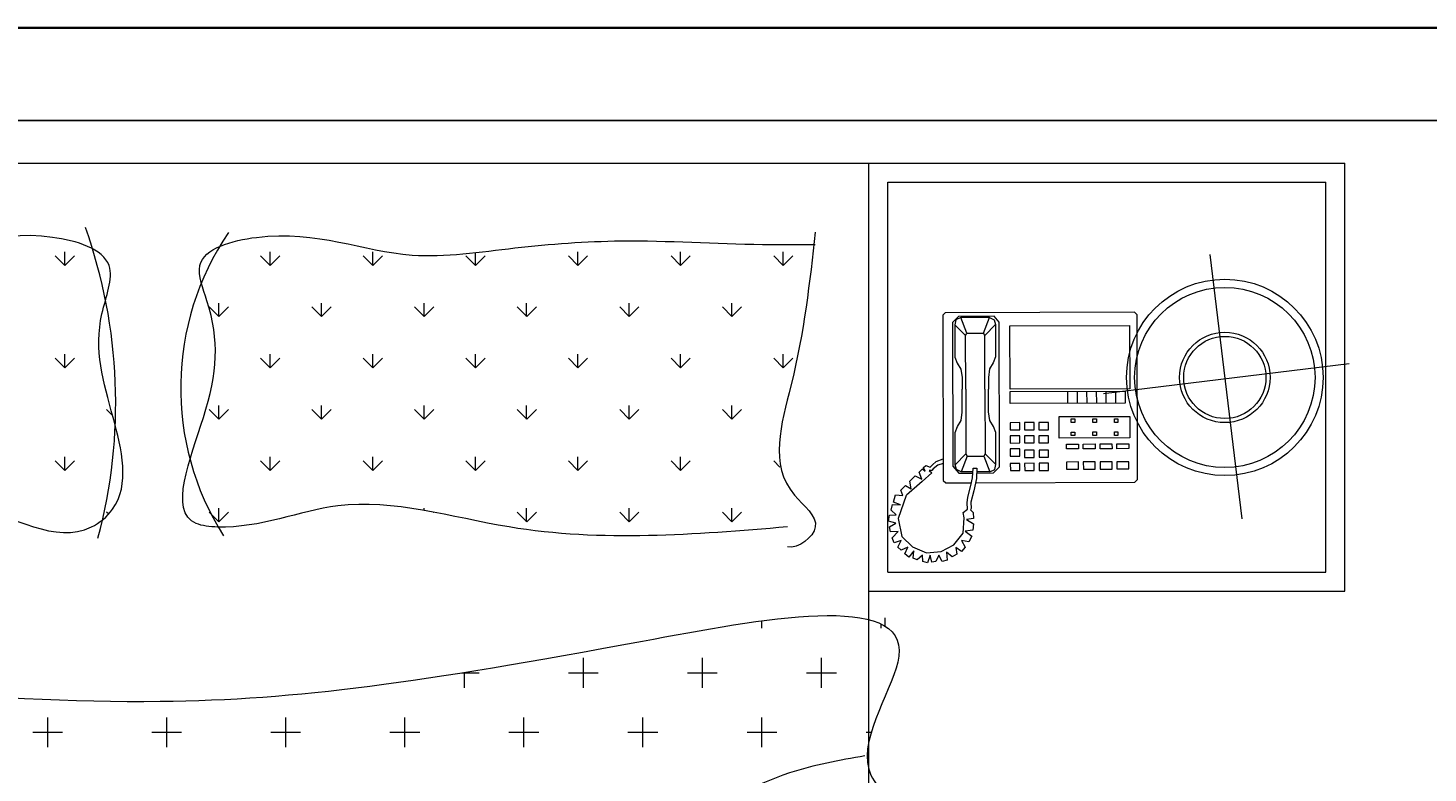
# Model space of a CAD drawing. Units: inches. Extents: x 3731 to 4318, y 1310 to 2388.
# Tile 29 of 57: x 3894 to 3954, y 1906 to 1938. Entities that reach past the tile are written whole.
import ezdxf

# ---------------------------------------------------------------- set-up
doc = ezdxf.new("R2010")
doc.units = ezdxf.units.IN
for name, color, linetype, lineweight in [('A-ANNO-DIMS', 2, 'Continuous', 18), ('A-FURN', 8, 'Continuous', 13), ('A-WALL', 7, 'Continuous', 35)]:
    doc.layers.add(name, color=color, linetype=linetype, lineweight=lineweight)
doc.styles.get("Standard").update_dxf_attribs({"font": 'arial.ttf'})
doc.dimstyles.get("Standard").update_dxf_attribs({"dimtxt": 0.18, "dimasz": 0.18, "dimexe": 0.18, "dimexo": 0.0625, "dimgap": 0.09, "dimtad": 0, "dimtih": 1, "dimtoh": 1, "dimdec": 4, "dimzin": 0, "dimdsep": 46, "dimtxsty": 'Standard', "dimcen": 0.09, "dimadec": 0, "dimazin": 0, "dimtfac": 1, "dimtdec": 4, "dimtofl": 0, "dimtmove": 0, "dimatfit": 3, "dimfxl": 1, "dimtolj": 1, "dimtzin": 0, "dimarcsym": 0})

# ---------------------------------------------------------------- blocks, each defined once
blk = doc.blocks.new('A$C200C7901')
for p, q in [((0.5, 2.3334), (2, 2.3334)), ((2, 2.3334), (2.5, 2.3334)), ((2, 1.6055), (2, 2.3334)), ((2.5, 1.8834), (2.5, 2.3334)), ((1.3176, 2.1721), (1.3075, 2.1822)), ((1.3176, 2.1721), (1.3075, 2.1822)), ((1.206, 2.0681), (1.1997, 2.0744)), ((1.206, 2.0681), (1.1997, 2.0744)), ((1.2019, 1.9645), (1.1997, 1.9666)), ((1.2019, 1.9645), (1.1997, 1.9666)), ((2, 1.8834), (2.5, 1.8834)), ((2.0171, 1.8467), (2.0171, 1.8556)), ((2.0171, 1.8467), (2.0171, 1.8556)), ((2.0129, 1.8445), (2.0129, 1.849)), ((2.0129, 1.8445), (2.0129, 1.849)), ((1.1379, 1.7195), (1.1379, 1.7508)), ((1.1222, 1.7352), (1.1535, 1.7352)), ((1.9972, 1.7352), (2.0027, 1.7352)), ((1.9972, 1.7352), (2.0027, 1.7352)), ((2, 1.6963), (2, 1.7248)), ((2, 1.6963), (2, 1.7248))]:
    blk.add_line(p, q)
at = {"linetype": 'ByBlock'}
for p, q in [((2.02, 2.3134), (2.48, 2.3134)), ((2.02, 1.9034), (2.02, 2.3134)), ((2.48, 1.9034), (2.48, 2.3134)), ((1.1559, 2.2259), (1.1458, 2.236)), ((1.1559, 2.2259), (1.1458, 2.236)), ((1.1559, 2.2259), (1.1559, 2.2402)), ((1.1559, 2.2259), (1.1559, 2.2402)), ((1.1559, 2.2259), (1.166, 2.236)), ((1.1559, 2.2259), (1.166, 2.236)), ((1.3714, 2.2259), (1.3613, 2.236)), ((1.3714, 2.2259), (1.3613, 2.236)), ((1.3714, 2.2259), (1.3714, 2.2402)), ((1.3714, 2.2259), (1.3714, 2.2402)), ((1.3714, 2.2259), (1.3815, 2.236)), ((1.3714, 2.2259), (1.3815, 2.236)), ((1.4792, 2.2259), (1.4691, 2.236)), ((1.4792, 2.2259), (1.4691, 2.236)), ((1.4792, 2.2259), (1.4792, 2.2402)), ((1.4792, 2.2259), (1.4792, 2.2402)), ((1.4792, 2.2259), (1.4893, 2.236)), ((1.4792, 2.2259), (1.4893, 2.236)), ((1.587, 2.2259), (1.5769, 2.236)), ((1.587, 2.2259), (1.5769, 2.236)), ((1.587, 2.2259), (1.587, 2.2393)), ((1.587, 2.2259), (1.587, 2.2393)), ((1.587, 2.2259), (1.5971, 2.236)), ((1.587, 2.2259), (1.5971, 2.236)), ((1.6947, 2.2259), (1.6846, 2.236)), ((1.6947, 2.2259), (1.6846, 2.236)), ((1.6947, 2.2259), (1.6947, 2.2402)), ((1.6947, 2.2259), (1.6947, 2.2402)), ((1.6947, 2.2259), (1.7048, 2.236)), ((1.6947, 2.2259), (1.7048, 2.236)), ((1.8025, 2.2259), (1.7924, 2.236)), ((1.8025, 2.2259), (1.7924, 2.236)), ((1.8025, 2.2259), (1.8025, 2.2402)), ((1.8025, 2.2259), (1.8025, 2.2402)), ((1.8025, 2.2259), (1.8126, 2.236)), ((1.8025, 2.2259), (1.8126, 2.236)), ((1.9103, 2.2259), (1.9002, 2.236)), ((1.9103, 2.2259), (1.9002, 2.236)), ((1.9103, 2.2259), (1.9103, 2.2402)), ((1.9103, 2.2259), (1.9103, 2.2402)), ((1.9103, 2.2259), (1.9204, 2.236)), ((1.9103, 2.2259), (1.9204, 2.236)), ((2.3581, 2.2373), (2.3919, 1.9595)), ((1.3176, 2.172), (1.3176, 2.1863)), ((1.3176, 2.172), (1.3176, 2.1863)), ((1.3176, 2.1721), (1.3277, 2.1822)), ((1.3176, 2.1721), (1.3277, 2.1822)), ((1.4253, 2.1721), (1.4152, 2.1822)), ((1.4253, 2.1721), (1.4152, 2.1822)), ((1.4253, 2.172), (1.4253, 2.1863)), ((1.4253, 2.172), (1.4253, 2.1863)), ((1.4253, 2.1721), (1.4354, 2.1822)), ((1.4253, 2.1721), (1.4354, 2.1822)), ((1.5331, 2.1721), (1.523, 2.1822)), ((1.5331, 2.1721), (1.523, 2.1822)), ((1.5331, 2.172), (1.5331, 2.1863)), ((1.5331, 2.172), (1.5331, 2.1863)), ((1.5331, 2.1721), (1.5432, 2.1822)), ((1.5331, 2.1721), (1.5432, 2.1822)), ((1.6409, 2.1721), (1.6308, 2.1822)), ((1.6409, 2.1721), (1.6308, 2.1822)), ((1.6408, 2.172), (1.6408, 2.1863)), ((1.6408, 2.172), (1.6408, 2.1863)), ((1.6409, 2.1721), (1.651, 2.1822)), ((1.6409, 2.1721), (1.651, 2.1822)), ((1.7486, 2.1721), (1.7385, 2.1822)), ((1.7486, 2.1721), (1.7385, 2.1822)), ((1.7486, 2.172), (1.7486, 2.1863)), ((1.7486, 2.172), (1.7486, 2.1863)), ((1.7486, 2.1721), (1.7587, 2.1822)), ((1.7486, 2.1721), (1.7587, 2.1822)), ((1.8564, 2.1721), (1.8463, 2.1822)), ((1.8564, 2.1721), (1.8463, 2.1822)), ((1.8564, 2.172), (1.8564, 2.1863)), ((1.8564, 2.172), (1.8564, 2.1863)), ((1.8564, 2.1721), (1.8665, 2.1822)), ((1.8564, 2.1721), (1.8665, 2.1822)), ((2.0802, 2.176), (2.0777, 2.1734)), ((2.2789, 2.1766), (2.0802, 2.176)), ((2.2789, 2.1766), (2.2814, 2.1741)), ((2.0777, 2.1734), (2.0783, 1.9999)), ((2.0941, 2.1722), (2.0878, 2.1659)), ((2.0878, 2.1659), (2.0883, 2.015)), ((2.0915, 2.1685), (2.0903, 2.1634)), ((2.0903, 2.1634), (2.1017, 2.1521)), ((2.0903, 2.1634), (2.0904, 2.1295)), ((2.0966, 2.171), (2.0915, 2.1685)), ((2.1318, 2.1724), (2.0941, 2.1722)), ((2.1267, 2.1711), (2.0966, 2.171)), ((2.1029, 2.1547), (2.0966, 2.171)), ((2.1205, 2.1547), (2.1267, 2.1711)), ((2.1331, 2.1636), (2.1218, 2.1522)), ((2.1267, 2.1711), (2.1318, 2.1686)), ((2.1368, 2.1661), (2.1318, 2.1724)), ((2.1318, 2.1686), (2.1331, 2.1636)), ((2.1331, 2.1636), (2.1332, 2.1296)), ((2.1373, 2.014), (2.1368, 2.1661)), ((2.1481, 2.1624), (2.2739, 2.1628)), ((2.1484, 2.0957), (2.1481, 2.1624)), ((2.2739, 2.1628), (2.2741, 2.0961)), ((2.2814, 2.1741), (2.282, 2.0006)), ((2.1017, 2.1521), (2.1029, 2.1547)), ((2.1019, 2.0956), (2.1017, 2.1521)), ((2.1029, 2.1547), (2.1205, 2.1547)), ((2.1218, 2.1522), (2.1205, 2.1547)), ((2.122, 2.0956), (2.1218, 2.1522)), ((1.1559, 2.1182), (1.1559, 2.1325)), ((1.1559, 2.1182), (1.1559, 2.1325)), ((1.3714, 2.1182), (1.3714, 2.1325)), ((1.3714, 2.1182), (1.3714, 2.1325)), ((1.4792, 2.1182), (1.4792, 2.1325)), ((1.4792, 2.1182), (1.4792, 2.1325)), ((1.587, 2.1182), (1.587, 2.1325)), ((1.587, 2.1182), (1.587, 2.1325)), ((1.6947, 2.1182), (1.6947, 2.1325)), ((1.6947, 2.1182), (1.6947, 2.1325)), ((1.8025, 2.1182), (1.8025, 2.1325)), ((1.8025, 2.1182), (1.8025, 2.1325)), ((1.9103, 2.1182), (1.9103, 2.1325)), ((1.9103, 2.1182), (1.9103, 2.1325)), ((1.1559, 2.1182), (1.1458, 2.1283)), ((1.1559, 2.1182), (1.1458, 2.1283)), ((1.1559, 2.1182), (1.166, 2.1283)), ((1.1559, 2.1182), (1.166, 2.1283)), ((1.3714, 2.1182), (1.3613, 2.1283)), ((1.3714, 2.1182), (1.3613, 2.1283)), ((1.3714, 2.1182), (1.3815, 2.1283)), ((1.3714, 2.1182), (1.3815, 2.1283)), ((1.4792, 2.1182), (1.4691, 2.1283)), ((1.4792, 2.1182), (1.4691, 2.1283)), ((1.4792, 2.1182), (1.4893, 2.1283)), ((1.4792, 2.1182), (1.4893, 2.1283)), ((1.587, 2.1182), (1.5769, 2.1283)), ((1.587, 2.1182), (1.5769, 2.1283)), ((1.587, 2.1182), (1.5971, 2.1283)), ((1.587, 2.1182), (1.5971, 2.1283)), ((1.6947, 2.1182), (1.6846, 2.1283)), ((1.6947, 2.1182), (1.6846, 2.1283)), ((1.6947, 2.1182), (1.7048, 2.1283)), ((1.6947, 2.1182), (1.7048, 2.1283)), ((1.8025, 2.1182), (1.7924, 2.1283)), ((1.8025, 2.1182), (1.7924, 2.1283)), ((1.8025, 2.1182), (1.8126, 2.1283)), ((1.8025, 2.1182), (1.8126, 2.1283)), ((1.9103, 2.1182), (1.9002, 2.1283)), ((1.9103, 2.1182), (1.9002, 2.1283)), ((1.9103, 2.1182), (1.9204, 2.1283)), ((1.9103, 2.1182), (1.9204, 2.1283)), ((2.0904, 2.1295), (2.093, 2.1232)), ((2.093, 2.1232), (2.0968, 2.1169)), ((2.0968, 2.1169), (2.098, 2.1081)), ((2.1269, 2.117), (2.1257, 2.1082)), ((2.1307, 2.1233), (2.1269, 2.117)), ((2.1332, 2.1296), (2.1307, 2.1233)), ((2.2464, 2.0911), (2.5044, 2.1228)), ((2.098, 2.1081), (2.0981, 2.0956)), ((2.1257, 2.1082), (2.1257, 2.0956)), ((2.0982, 2.0717), (2.0981, 2.0956)), ((2.1019, 2.0956), (2.1021, 2.0277)), ((2.122, 2.0956), (2.1222, 2.0277)), ((2.1258, 2.0718), (2.1257, 2.0956)), ((2.2741, 2.0961), (2.1484, 2.0957)), ((2.1484, 2.0932), (2.2691, 2.0936)), ((2.1484, 2.0806), (2.1484, 2.0932)), ((2.2087, 2.0934), (2.2088, 2.0808)), ((2.2188, 2.0934), (2.2188, 2.0809)), ((2.2288, 2.0935), (2.2289, 2.0809)), ((2.2389, 2.0935), (2.239, 2.0809)), ((2.249, 2.0935), (2.249, 2.081)), ((2.259, 2.0936), (2.2591, 2.081)), ((2.2691, 2.0936), (2.2691, 2.081)), ((1.3176, 2.0643), (1.3075, 2.0744)), ((1.3176, 2.0643), (1.3075, 2.0744)), ((1.3176, 2.0643), (1.3176, 2.0786)), ((1.3176, 2.0643), (1.3176, 2.0786)), ((1.3176, 2.0643), (1.3277, 2.0744)), ((1.3176, 2.0643), (1.3277, 2.0744)), ((1.4253, 2.0643), (1.4152, 2.0744)), ((1.4253, 2.0643), (1.4152, 2.0744)), ((1.4253, 2.0643), (1.4253, 2.0786)), ((1.4253, 2.0643), (1.4253, 2.0786)), ((1.4253, 2.0643), (1.4354, 2.0744)), ((1.4253, 2.0643), (1.4354, 2.0744)), ((1.5331, 2.0643), (1.523, 2.0744)), ((1.5331, 2.0643), (1.523, 2.0744)), ((1.5331, 2.0643), (1.5331, 2.0786)), ((1.5331, 2.0643), (1.5331, 2.0786)), ((1.5331, 2.0643), (1.5432, 2.0744)), ((1.5331, 2.0643), (1.5432, 2.0744)), ((1.6409, 2.0643), (1.6308, 2.0744)), ((1.6409, 2.0643), (1.6308, 2.0744)), ((1.6408, 2.0643), (1.6408, 2.0786)), ((1.6408, 2.0643), (1.6408, 2.0786)), ((1.6409, 2.0643), (1.651, 2.0744)), ((1.6409, 2.0643), (1.651, 2.0744)), ((1.7486, 2.0643), (1.7385, 2.0744)), ((1.7486, 2.0643), (1.7385, 2.0744)), ((1.7486, 2.0643), (1.7486, 2.0786)), ((1.7486, 2.0643), (1.7486, 2.0786)), ((1.7486, 2.0643), (1.7587, 2.0744)), ((1.7486, 2.0643), (1.7587, 2.0744)), ((1.8564, 2.0643), (1.8463, 2.0744)), ((1.8564, 2.0643), (1.8463, 2.0744)), ((1.8564, 2.0643), (1.8564, 2.0786)), ((1.8564, 2.0643), (1.8564, 2.0786)), ((1.8564, 2.0643), (1.8665, 2.0744)), ((1.8564, 2.0643), (1.8665, 2.0744)), ((2.2691, 2.081), (2.1484, 2.0806)), ((2.0932, 2.0566), (2.0969, 2.0629)), ((2.0969, 2.0629), (2.0982, 2.0717)), ((2.1271, 2.063), (2.1258, 2.0718)), ((2.1309, 2.0567), (2.1271, 2.063)), ((2.1586, 2.0606), (2.1485, 2.0605)), ((2.1485, 2.0605), (2.1485, 2.053)), ((2.1586, 2.053), (2.1586, 2.0606)), ((2.1636, 2.0606), (2.1636, 2.053)), ((2.1736, 2.0606), (2.1636, 2.0606)), ((2.1737, 2.0531), (2.1736, 2.0606)), ((2.1887, 2.0607), (2.1787, 2.0606)), ((2.1787, 2.0606), (2.1787, 2.0531)), ((2.1888, 2.0531), (2.1887, 2.0607)), ((2.2, 2.067), (2.2742, 2.0672)), ((2.2001, 2.0443), (2.2, 2.067)), ((2.2126, 2.0645), (2.2164, 2.0645)), ((2.2126, 2.0607), (2.2126, 2.0645)), ((2.2164, 2.0607), (2.2126, 2.0607)), ((2.2164, 2.0645), (2.2164, 2.0607)), ((2.2352, 2.0646), (2.239, 2.0646)), ((2.2352, 2.0608), (2.2352, 2.0646)), ((2.239, 2.0608), (2.2352, 2.0608)), ((2.239, 2.0646), (2.239, 2.0608)), ((2.2579, 2.0609), (2.2579, 2.0647)), ((2.2579, 2.0647), (2.2616, 2.0647)), ((2.2616, 2.0609), (2.2579, 2.0609)), ((2.2616, 2.0647), (2.2616, 2.0609)), ((2.2742, 2.0672), (2.2743, 2.0446)), ((2.0907, 2.0503), (2.0932, 2.0566)), ((2.0908, 2.0163), (2.0907, 2.0503)), ((2.1334, 2.0504), (2.1309, 2.0567)), ((2.1336, 2.0165), (2.1334, 2.0504)), ((2.1485, 2.053), (2.1586, 2.053)), ((2.1485, 2.0467), (2.1486, 2.0391)), ((2.1586, 2.0467), (2.1485, 2.0467)), ((2.1586, 2.0392), (2.1586, 2.0467)), ((2.1636, 2.053), (2.1737, 2.0531)), ((2.1737, 2.0468), (2.1636, 2.0467)), ((2.1636, 2.0467), (2.1637, 2.0392)), ((2.1737, 2.0392), (2.1737, 2.0468)), ((2.1787, 2.0531), (2.1888, 2.0531)), ((2.1787, 2.0468), (2.1787, 2.0392)), ((2.1888, 2.0468), (2.1787, 2.0468)), ((2.1888, 2.0393), (2.1888, 2.0468)), ((2.2743, 2.0446), (2.2001, 2.0443)), ((2.2126, 2.0507), (2.2164, 2.0507)), ((2.2127, 2.0469), (2.2126, 2.0507)), ((2.2164, 2.0469), (2.2127, 2.0469)), ((2.2164, 2.0507), (2.2164, 2.0469)), ((2.2353, 2.0508), (2.2391, 2.0508)), ((2.2353, 2.047), (2.2353, 2.0508)), ((2.2391, 2.047), (2.2353, 2.047)), ((2.2391, 2.0508), (2.2391, 2.047)), ((2.2579, 2.0508), (2.2617, 2.0508)), ((2.2579, 2.0471), (2.2579, 2.0508)), ((2.2617, 2.0471), (2.2579, 2.0471)), ((2.2617, 2.0508), (2.2617, 2.0471)), ((2.1486, 2.0391), (2.1586, 2.0392)), ((2.1586, 2.0329), (2.1486, 2.0329)), ((2.1486, 2.0329), (2.1486, 2.0253)), ((2.1587, 2.0253), (2.1586, 2.0329)), ((2.1637, 2.0392), (2.1737, 2.0392)), ((2.1637, 2.0317), (2.1637, 2.0241)), ((2.1737, 2.0317), (2.1637, 2.0317)), ((2.1738, 2.0241), (2.1737, 2.0317)), ((2.1787, 2.0392), (2.1888, 2.0393)), ((2.1788, 2.0317), (2.1788, 2.0242)), ((2.1888, 2.0317), (2.1788, 2.0317)), ((2.1889, 2.0242), (2.1888, 2.0317)), ((2.2077, 2.0331), (2.2077, 2.0381)), ((2.2077, 2.0381), (2.2202, 2.0381)), ((2.2203, 2.0331), (2.2077, 2.0331)), ((2.2202, 2.0381), (2.2203, 2.0331)), ((2.2253, 2.0381), (2.2378, 2.0382)), ((2.2253, 2.0331), (2.2253, 2.0381)), ((2.2379, 2.0332), (2.2253, 2.0331)), ((2.2378, 2.0382), (2.2379, 2.0332)), ((2.2429, 2.0332), (2.2429, 2.0382)), ((2.2429, 2.0382), (2.2554, 2.0382)), ((2.2555, 2.0332), (2.2429, 2.0332)), ((2.2554, 2.0382), (2.2555, 2.0332)), ((2.2605, 2.0332), (2.2605, 2.0383)), ((2.2605, 2.0383), (2.273, 2.0383)), ((2.2731, 2.0333), (2.2605, 2.0332)), ((2.273, 2.0383), (2.2731, 2.0333)), ((1.1559, 2.0104), (1.1458, 2.0205)), ((1.1559, 2.0104), (1.1458, 2.0205)), ((1.1559, 2.0104), (1.1559, 2.0247)), ((1.1559, 2.0104), (1.1559, 2.0247)), ((1.1559, 2.0104), (1.166, 2.0205)), ((1.1559, 2.0104), (1.166, 2.0205)), ((1.3714, 2.0104), (1.3613, 2.0205)), ((1.3714, 2.0104), (1.3613, 2.0205)), ((1.3714, 2.0104), (1.3714, 2.0247)), ((1.3714, 2.0104), (1.3714, 2.0247)), ((1.3714, 2.0104), (1.3815, 2.0205)), ((1.3714, 2.0104), (1.3815, 2.0205)), ((1.4792, 2.0104), (1.4691, 2.0205)), ((1.4792, 2.0104), (1.4691, 2.0205)), ((1.4792, 2.0104), (1.4792, 2.0247)), ((1.4792, 2.0104), (1.4792, 2.0247)), ((1.4792, 2.0104), (1.4893, 2.0205)), ((1.4792, 2.0104), (1.4893, 2.0205)), ((1.587, 2.0104), (1.5769, 2.0205)), ((1.587, 2.0104), (1.5769, 2.0205)), ((1.587, 2.0104), (1.587, 2.0247)), ((1.587, 2.0104), (1.587, 2.0247)), ((1.587, 2.0104), (1.5971, 2.0205)), ((1.587, 2.0104), (1.5971, 2.0205)), ((1.6947, 2.0104), (1.6846, 2.0205)), ((1.6947, 2.0104), (1.6846, 2.0205)), ((1.6947, 2.0104), (1.6947, 2.0247)), ((1.6947, 2.0104), (1.6947, 2.0247)), ((1.6947, 2.0104), (1.7048, 2.0205)), ((1.6947, 2.0104), (1.7048, 2.0205)), ((1.8025, 2.0104), (1.7924, 2.0205)), ((1.8025, 2.0104), (1.7924, 2.0205)), ((1.8025, 2.0104), (1.8025, 2.0247)), ((1.8025, 2.0104), (1.8025, 2.0247)), ((1.8025, 2.0104), (1.8126, 2.0205)), ((1.8025, 2.0104), (1.8126, 2.0205)), ((1.9068, 2.0139), (1.9002, 2.0205)), ((1.9068, 2.0139), (1.9002, 2.0205)), ((2.0576, 2.0133), (2.0598, 2.0155)), ((2.0598, 2.0155), (2.0645, 2.0137)), ((2.0645, 2.0137), (2.0671, 2.0162)), ((2.0671, 2.0162), (2.0707, 2.0197)), ((2.0727, 2.016), (2.0676, 2.012)), ((2.0707, 2.0197), (2.0782, 2.0226)), ((2.0782, 2.0175), (2.0727, 2.016)), ((2.0883, 2.015), (2.0946, 2.0075)), ((2.0908, 2.0163), (2.1021, 2.0277)), ((2.0921, 2.0113), (2.0908, 2.0163)), ((2.1034, 2.0252), (2.0971, 2.0088)), ((2.1021, 2.0277), (2.1034, 2.0252)), ((2.1034, 2.0252), (2.121, 2.0252)), ((2.1222, 2.0277), (2.121, 2.0252)), ((2.121, 2.0252), (2.1273, 2.0089)), ((2.1336, 2.0165), (2.1222, 2.0277)), ((2.1323, 2.0114), (2.1336, 2.0165)), ((2.1486, 2.0253), (2.1587, 2.0253)), ((2.1587, 2.0178), (2.1486, 2.0178)), ((2.1486, 2.0178), (2.1487, 2.0102)), ((2.1587, 2.0103), (2.1587, 2.0178)), ((2.1637, 2.0241), (2.1738, 2.0241)), ((2.1738, 2.0179), (2.1637, 2.0178)), ((2.1637, 2.0178), (2.1638, 2.0103)), ((2.1738, 2.0103), (2.1738, 2.0179)), ((2.1788, 2.0242), (2.1889, 2.0242)), ((2.1788, 2.0179), (2.1788, 2.0103)), ((2.1889, 2.0179), (2.1788, 2.0179)), ((2.1889, 2.0104), (2.1889, 2.0179)), ((2.2203, 2.0193), (2.2077, 2.0192)), ((2.2077, 2.0192), (2.2078, 2.0117)), ((2.2203, 2.0117), (2.2203, 2.0193)), ((2.2379, 2.0193), (2.2253, 2.0193)), ((2.2253, 2.0193), (2.2254, 2.0117)), ((2.2379, 2.0118), (2.2379, 2.0193)), ((2.2555, 2.0194), (2.2429, 2.0193)), ((2.2429, 2.0193), (2.243, 2.0118)), ((2.2555, 2.0118), (2.2555, 2.0194)), ((2.2605, 2.0194), (2.2606, 2.0119)), ((2.2731, 2.0194), (2.2605, 2.0194)), ((2.2731, 2.0119), (2.2731, 2.0194)), ((2.0431, 1.999), (2.0488, 2.0046)), ((2.0488, 2.0046), (2.0557, 2.0011)), ((2.053, 2.0084), (2.0563, 2.0119)), ((2.0557, 2.0011), (2.053, 2.0084)), ((2.0663, 2.0077), (2.0561, 1.9986)), ((2.0563, 2.0119), (2.0594, 2.0095)), ((2.0594, 2.0095), (2.0576, 2.0133)), ((2.0663, 2.0102), (2.0636, 2.0104)), ((2.0636, 2.0104), (2.0663, 2.0077)), ((2.0676, 2.012), (2.0663, 2.0102)), ((2.0783, 1.9999), (2.0808, 1.9974)), ((2.0971, 2.0088), (2.0921, 2.0113)), ((2.0946, 2.0075), (2.1093, 2.0076)), ((2.1094, 2.0088), (2.0971, 2.0088)), ((2.1072, 1.9944), (2.109, 2.0025)), ((2.109, 2.0025), (2.1097, 2.0126)), ((2.1097, 2.0126), (2.1135, 2.0126)), ((2.1133, 2.0018), (2.1103, 1.989)), ((2.1135, 2.0126), (2.1133, 2.0018)), ((2.1273, 2.0089), (2.1134, 2.0088)), ((2.1134, 2.0076), (2.1311, 2.0077)), ((2.1273, 2.0089), (2.1323, 2.0114)), ((2.1311, 2.0077), (2.1373, 2.014)), ((2.1487, 2.0102), (2.1587, 2.0103)), ((2.1638, 2.0103), (2.1738, 2.0103)), ((2.1788, 2.0103), (2.1889, 2.0104)), ((2.2078, 2.0117), (2.2203, 2.0117)), ((2.2254, 2.0117), (2.2379, 2.0118)), ((2.243, 2.0118), (2.2555, 2.0118)), ((2.2606, 2.0119), (2.2731, 2.0119)), ((2.282, 2.0006), (2.2795, 1.9981)), ((2.0259, 1.977), (2.0281, 1.9847)), ((2.0281, 1.9847), (2.0358, 1.9839)), ((2.0338, 1.9895), (2.0386, 1.9946)), ((2.0358, 1.9839), (2.0338, 1.9895)), ((2.0386, 1.9946), (2.0444, 1.9911)), ((2.0561, 1.9986), (2.0396, 1.9844)), ((2.0444, 1.9911), (2.0431, 1.999)), ((2.0808, 1.9974), (2.1079, 1.9975)), ((2.1042, 1.9824), (2.1072, 1.9944)), ((2.1103, 1.989), (2.1073, 1.9771)), ((2.1123, 1.9975), (2.2795, 1.9981)), ((1.3176, 1.9565), (1.3176, 1.9708)), ((1.3176, 1.9565), (1.3176, 1.9708)), ((1.4253, 1.9703), (1.4253, 1.9708)), ((1.4253, 1.9703), (1.4253, 1.9708)), ((1.5331, 1.9683), (1.5331, 1.9708)), ((1.5331, 1.9683), (1.5331, 1.9708)), ((1.6408, 1.9565), (1.6408, 1.9708)), ((1.6408, 1.9565), (1.6408, 1.9708)), ((1.7486, 1.9565), (1.7486, 1.9708)), ((1.7486, 1.9565), (1.7486, 1.9708)), ((1.8564, 1.9565), (1.8564, 1.9708)), ((1.8564, 1.9565), (1.8564, 1.9708)), ((2.0234, 1.9686), (2.0251, 1.9745)), ((2.0251, 1.9745), (2.0333, 1.9743)), ((2.0333, 1.9743), (2.0259, 1.977)), ((2.0393, 1.984), (2.031, 1.96)), ((2.1035, 1.9763), (2.1042, 1.9824)), ((2.1038, 1.9697), (2.1035, 1.9763)), ((2.1076, 1.9704), (2.1068, 1.9689)), ((2.1073, 1.9771), (2.1076, 1.9704)), ((1.3176, 1.9565), (1.3075, 1.9666)), ((1.3176, 1.9565), (1.3075, 1.9666)), ((1.3176, 1.9565), (1.3277, 1.9666)), ((1.3176, 1.9565), (1.3277, 1.9666)), ((1.543, 1.9665), (1.5432, 1.9666)), ((1.543, 1.9665), (1.5432, 1.9666)), ((1.6409, 1.9565), (1.6308, 1.9666)), ((1.6409, 1.9565), (1.6308, 1.9666)), ((1.6409, 1.9565), (1.651, 1.9666)), ((1.6409, 1.9565), (1.651, 1.9666)), ((1.7486, 1.9565), (1.7385, 1.9666)), ((1.7486, 1.9565), (1.7385, 1.9666)), ((1.7486, 1.9565), (1.7587, 1.9666)), ((1.7486, 1.9565), (1.7587, 1.9666)), ((1.8564, 1.9565), (1.8463, 1.9666)), ((1.8564, 1.9565), (1.8463, 1.9666)), ((1.8564, 1.9565), (1.8665, 1.9666)), ((1.8564, 1.9565), (1.8665, 1.9666)), ((2.0206, 1.9572), (2.0218, 1.9635)), ((2.0285, 1.9549), (2.0206, 1.9572)), ((2.0218, 1.9635), (2.0287, 1.9636)), ((2.0287, 1.9636), (2.0234, 1.9686)), ((2.031, 1.96), (2.0346, 1.9409)), ((2.099, 1.9444), (2.1002, 1.9605)), ((2.0992, 1.9663), (2.1038, 1.9697)), ((2.1002, 1.9605), (2.0992, 1.9663)), ((2.1101, 1.96), (2.1028, 1.9587)), ((2.1028, 1.9587), (2.1099, 1.9544)), ((2.1068, 1.9689), (2.1096, 1.9661)), ((2.1096, 1.9661), (2.1101, 1.96)), ((2.0219, 1.9511), (2.0285, 1.9549)), ((2.0229, 1.946), (2.0219, 1.9511)), ((2.0308, 1.9462), (2.0229, 1.946)), ((2.0247, 1.9394), (2.0308, 1.9462)), ((2.0346, 1.9409), (2.0459, 1.93)), ((2.0894, 1.9322), (2.099, 1.9444)), ((2.1094, 1.9475), (2.1013, 1.9467)), ((2.1013, 1.9467), (2.1084, 1.9412)), ((2.1084, 1.9412), (2.1051, 1.9353)), ((2.1099, 1.9544), (2.1094, 1.9475)), ((2.0268, 1.9343), (2.0247, 1.9394)), ((2.0341, 1.9366), (2.0268, 1.9343)), ((2.0306, 1.9297), (2.0341, 1.9366)), ((2.0339, 1.9267), (2.0306, 1.9297)), ((2.041, 1.9297), (2.0339, 1.9267)), ((2.038, 1.9228), (2.041, 1.9297)), ((2.0474, 1.9259), (2.0421, 1.9193)), ((2.0459, 1.93), (2.0607, 1.9237)), ((2.0467, 1.9183), (2.0474, 1.9259)), ((2.0759, 1.925), (2.0894, 1.9322)), ((2.0973, 1.9251), (2.0914, 1.9294)), ((2.0914, 1.9294), (2.0925, 1.9225)), ((2.1011, 1.9297), (2.0973, 1.9251)), ((2.1051, 1.9353), (2.0975, 1.9368)), ((2.0975, 1.9368), (2.1011, 1.9297)), ((2.0421, 1.9193), (2.038, 1.9228)), ((2.0508, 1.9163), (2.0467, 1.9183)), ((2.0566, 1.9214), (2.0508, 1.9163)), ((2.0569, 1.9145), (2.0566, 1.9214)), ((2.0617, 1.9133), (2.0569, 1.9145)), ((2.0607, 1.9237), (2.0759, 1.925)), ((2.0645, 1.9214), (2.0617, 1.9133)), ((2.0663, 1.914), (2.0645, 1.9214)), ((2.0706, 1.9146), (2.0663, 1.914)), ((2.0736, 1.9214), (2.0706, 1.9146)), ((2.077, 1.9146), (2.0736, 1.9214)), ((2.0823, 1.9161), (2.077, 1.9146)), ((2.0876, 1.9195), (2.0815, 1.9245)), ((2.0815, 1.9245), (2.0823, 1.9161)), ((2.0925, 1.9225), (2.0876, 1.9195)), ((2.02, 1.9034), (2.48, 1.9034)), ((1.8879, 1.8445), (1.8879, 1.8523)), ((1.8879, 1.8445), (1.8879, 1.8523)), ((1.7004, 1.782), (1.7004, 1.8133)), ((1.7004, 1.782), (1.7004, 1.8133)), ((1.8254, 1.782), (1.8254, 1.8133)), ((1.8254, 1.782), (1.8254, 1.8133)), ((1.9504, 1.782), (1.9504, 1.8133)), ((1.9504, 1.782), (1.9504, 1.8133)), ((1.573, 1.7977), (1.591, 1.7977)), ((1.573, 1.7977), (1.591, 1.7977)), ((1.5754, 1.782), (1.5754, 1.7981)), ((1.5754, 1.782), (1.5754, 1.7981)), ((1.6847, 1.7977), (1.716, 1.7977)), ((1.6847, 1.7977), (1.716, 1.7977)), ((1.8097, 1.7977), (1.841, 1.7977)), ((1.8097, 1.7977), (1.841, 1.7977)), ((1.9347, 1.7977), (1.966, 1.7977)), ((1.9347, 1.7977), (1.966, 1.7977)), ((1.1379, 1.7195), (1.1379, 1.7508)), ((1.2629, 1.7195), (1.2629, 1.7508)), ((1.2629, 1.7195), (1.2629, 1.7508)), ((1.3879, 1.7195), (1.3879, 1.7508)), ((1.3879, 1.7195), (1.3879, 1.7508)), ((1.5129, 1.7195), (1.5129, 1.7508)), ((1.5129, 1.7195), (1.5129, 1.7508)), ((1.6379, 1.7195), (1.6379, 1.7508)), ((1.6379, 1.7195), (1.6379, 1.7508)), ((1.7629, 1.7195), (1.7629, 1.7508)), ((1.7629, 1.7195), (1.7629, 1.7508)), ((1.8879, 1.7195), (1.8879, 1.7508)), ((1.8879, 1.7195), (1.8879, 1.7508)), ((1.1222, 1.7352), (1.1535, 1.7352)), ((1.2472, 1.7352), (1.2785, 1.7352)), ((1.2472, 1.7352), (1.2785, 1.7352)), ((1.3722, 1.7352), (1.4035, 1.7352)), ((1.3722, 1.7352), (1.4035, 1.7352)), ((1.4972, 1.7352), (1.5285, 1.7352)), ((1.4972, 1.7352), (1.5285, 1.7352)), ((1.6222, 1.7352), (1.6535, 1.7352)), ((1.6222, 1.7352), (1.6535, 1.7352)), ((1.7472, 1.7352), (1.7785, 1.7352)), ((1.7472, 1.7352), (1.7785, 1.7352)), ((1.8722, 1.7352), (1.9035, 1.7352)), ((1.8722, 1.7352), (1.9035, 1.7352))]:
    blk.add_line(p, q, dxfattribs=at)
for radius in [0.1032, 0.0947, 0.0475, 0.0432]:
    blk.add_circle((2.3739, 2.1081), radius, dxfattribs=at)
for centre, radius, start, end in [((0.658, 2.0811), 0.5513, 345.0722, 19.5492), ((1.5685, 2.097), 0.291, 145.8603, 212.2445)]:
    blk.add_arc(centre, radius, start, end)
for points, knots in [([(0.5854, 1.951), (0.6835, 1.9407), (0.8425, 1.9242), (1.0374, 2.0054), (1.1564, 1.9255), (1.2274, 1.9841), (1.2052, 2.0751), (1.1815, 2.152), (1.2176, 2.2368), (1.0992, 2.2731), (1.0008, 2.2255), (0.8698, 2.246), (0.7481, 2.2548), (0.6426, 2.2473), (0.5746, 2.2478), (0.5562, 2.2479)], [0, 0, 0, 0, 292.165466, 473.33038, 601.631673, 630.723769, 727.138505, 836.819956, 887.958136, 954.42438, 1118.989809, 1227.016542, 1338.750986, 1487.447361, 1542.751028, 1542.751028, 1542.751028, 1542.751028]), ([(1.9146, 1.951), (1.8174, 1.9428), (1.6601, 1.9297), (1.4574, 1.9942), (1.3549, 1.9462), (1.2593, 1.9563), (1.314, 2.0834), (1.3193, 2.1569), (1.2853, 2.2393), (1.4031, 2.2724), (1.4987, 2.2256), (1.6304, 2.2459), (1.7519, 2.2548), (1.8574, 2.2473), (1.9254, 2.2478), (1.9438, 2.2479)], [0, 0, 0, 0, 292.165466, 473.33038, 601.631673, 624.236147, 735.870502, 858.452188, 896.317728, 962.783971, 1127.3494, 1235.376134, 1347.110578, 1495.806953, 1551.11062, 1551.11062, 1551.11062, 1551.11062]), ([(1.9438, 2.2608), (1.9381, 2.2086), (1.9282, 2.1195), (1.8897, 2.0022), (1.9591, 1.9538), (1.9264, 1.9278), (1.9146, 1.93)], [0, 0, 0, 0, 163.411291, 278.570782, 318.445997, 354.484131, 354.484131, 354.484131, 354.484131]), ([(0.4485, 1.7835), (0.4321, 1.7496), (0.4062, 1.6964), (0.49, 1.6713), (0.4719, 1.5969), (0.4123, 1.592), (0.4233, 1.5337), (0.4954, 1.5086), (0.4012, 1.4738), (0.3253, 1.4306), (0.4113, 1.3764), (0.3688, 1.3065), (0.5579, 1.2663), (0.741, 1.4533), (1.1127, 1.1109), (1.4811, 1.2478), (1.7885, 1.3492), (2.0357, 1.1637), (2.0748, 1.2974), (2.0876, 1.349), (2.0192, 1.3805), (2.0564, 1.4298), (2.0588, 1.4846), (1.9759, 1.5349), (2.1004, 1.5845), (2.0397, 1.6519), (1.971, 1.7053), (2.1104, 1.8981), (1.5946, 1.7967), (1.2448, 1.7472), (0.8129, 1.7935), (0.4953, 1.8548), (0.4582, 1.7983), (0.4485, 1.7835)], [0, 0, 0, 0, 88.420092, 139.08588, 204.302936, 239.695496, 287.801042, 327.365471, 412.960499, 463.626286, 552.059846, 584.668336, 662.614915, 940.993281, 1309.926334, 1844.022653, 1996.276242, 2316.43048, 2341.441004, 2404.707416, 2449.463774, 2514.680778, 2538.40571, 2613.031547, 2697.13096, 2760.903931, 2822.692699, 2945.47, 3215.060018, 3725.584917, 4361.974444, 4504.671998, 4555.32777, 4555.32777, 4555.32777, 4555.32777])]:
    blk.add_open_spline(points, degree=3, knots=knots)
blk.add_open_spline([(1.996, 1.7104), (1.9692, 1.7057), (1.9025, 1.6938), (1.844, 1.6592), (1.809, 1.6385)], degree=3, knots=[0, 0, 0, 0, 81.132613, 201.738644, 201.738644, 201.738644, 201.738644], dxfattribs=at)
blk.add_open_spline([(1.996, 1.7104), (1.9692, 1.7057), (1.9025, 1.6938), (1.844, 1.6592), (1.809, 1.6385)], degree=3, knots=[0, 0, 0, 0, 81.132613, 201.738644, 201.738644, 201.738644, 201.738644], dxfattribs=at)
blk = doc.blocks.new('*D45')
at = {"layer": 'A-ANNO-DIMS', "color": 0, "lineweight": -2, "transparency": 16777216}
for p, q in [((3969.146, 1934.382), (3731.412, 1934.382)), ((3731.592, 1934.202), (3731.592, 1904.563)), ((3731.592, 1874.562), (3731.592, 1904.2)), ((3969.146, 1874.382), (3731.412, 1874.382))]:
    blk.add_line(p, q, dxfattribs=at)
at = {"layer": 'A-ANNO-DIMS', "color": 0, "transparency": 16777216}
for points in [[(3731.562, 1934.202), (3731.622, 1934.202), (3731.592, 1934.382)], [(3731.562, 1874.562), (3731.622, 1874.562), (3731.592, 1874.382)]]:
    blk.add_solid(points, dxfattribs=at)
at = {"layer": 'Defpoints', "color": 0, "transparency": 16777216}
for p in [(3731.592, 1934.382), (3969.209, 1934.382), (3969.209, 1874.382)]:
    blk.add_point(p, dxfattribs=at)
at = {"layer": 'A-ANNO-DIMS', "color": 0, "transparency": 16777216, "insert": (3731.592, 1904.382), "char_height": 0.18, "attachment_point": 5}
blk.add_mtext('\\A1;60', dxfattribs=at)

msp = doc.modelspace()

# ---------------------------------------------------------------- linework, layer by layer
at = {"layer": 'A-WALL'}
msp.add_line((3840.209, 1938.382), (3960.209, 1938.382), dxfattribs=at)

# ---------------------------------------------------------------- block references
at = {"layer": 'A-FURN', "xscale": 41.1071563136412, "yscale": 41.1071563136412, "zscale": 41.1071563136412}
msp.add_blockref('A$C200C7901', (3848.004, 1836.625), dxfattribs=at)

# ---------------------------------------------------------------- dimensions: what is measured, and where the dimension line sits
at = {"layer": 'A-ANNO-DIMS'}
dim = msp.add_linear_dim(base=(3731.592, 1934.382), p1=(3969.209, 1874.382), p2=(3969.209, 1934.382), angle=90, dimstyle='Standard', override={"dimdec": 0, "dimlfac": 1, "dimrnd": 0, "dimzin": 0, "dimdsep": 46, "dimlunit": 2}, dxfattribs=at)
dim.commit()
dim.dimension.update_dxf_attribs({"geometry": '*D45', "text_midpoint": (3731.592, 1904.382)})

doc.saveas('drawing.dxf')
